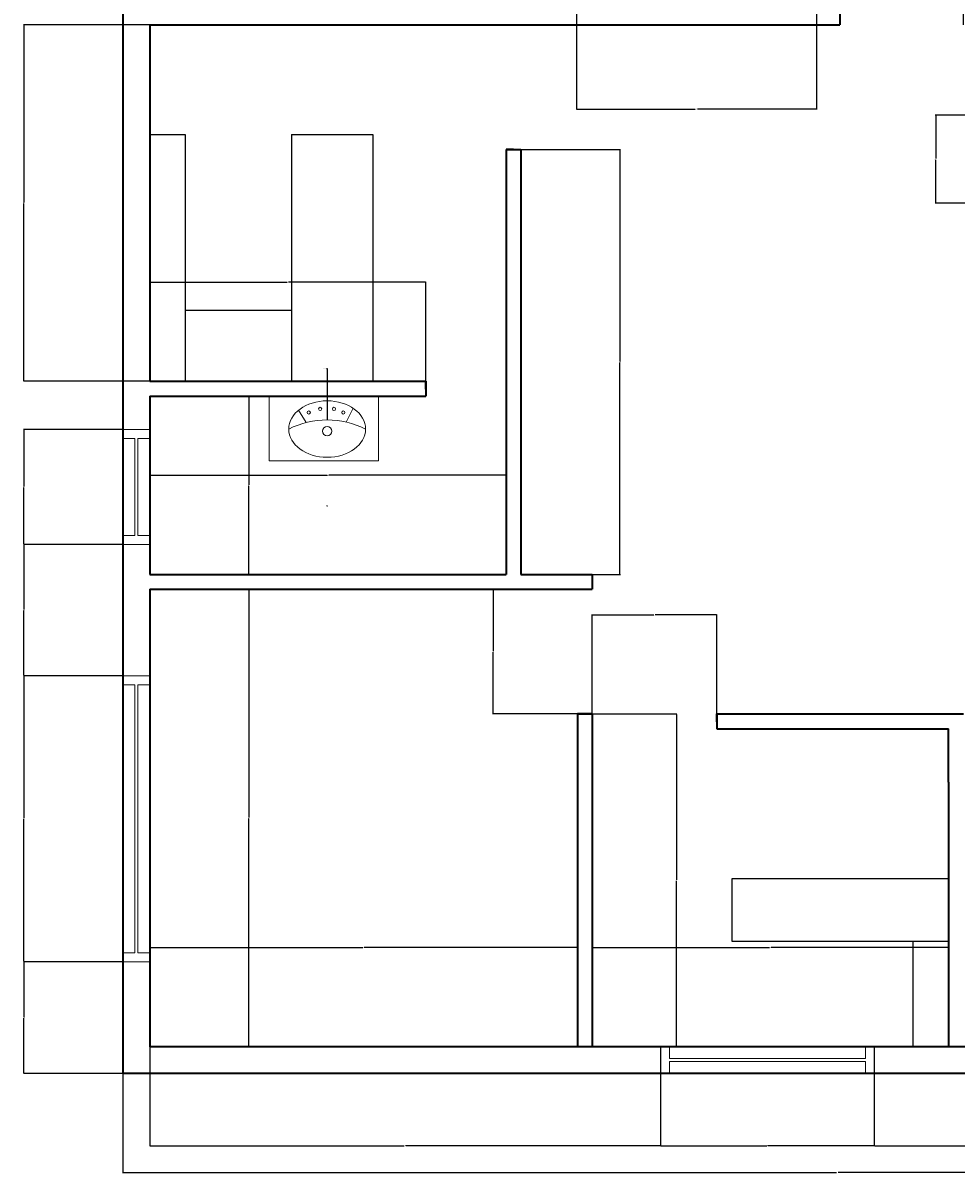
# Model space of a CAD drawing. Units: inches. Extents: x 1201 to 1750, y 1179 to 1858.
# Tile 1 of 3: x 1201 to 1515, y 1179 to 1566. Entities that reach past the tile are written whole.
import ezdxf

# ---------------------------------------------------------------- set-up
doc = ezdxf.new("R2010")
doc.units = ezdxf.units.IN
for name, color, linetype, lineweight in [('A-ANNO-DIMS', 2, 'Continuous', 18), ('A-FLOR-CASE', 9, 'Continuous', 25), ('A-FLOR-FIXT', 9, 'Continuous', 18), ('A-GLAZ', 4, 'Continuous', 18), ('A-WALL', 7, 'Continuous', 35)]:
    doc.layers.add(name, color=color, linetype=linetype, lineweight=lineweight)
doc.styles.get("Standard").update_dxf_attribs({"font": 'times.ttf'})
doc.dimstyles.get("Standard").update_dxf_attribs({"dimtxt": 0.18, "dimasz": 0.18, "dimexe": 0.18, "dimexo": 0.0625, "dimgap": 0.09, "dimtad": 0, "dimtih": 1, "dimtoh": 1, "dimdec": 4, "dimzin": 0, "dimdsep": 46, "dimtxsty": 'Standard', "dimcen": 0.09, "dimadec": 0, "dimazin": 0, "dimtfac": 1, "dimtdec": 4, "dimtofl": 0, "dimtmove": 0, "dimatfit": 3, "dimfxl": 1, "dimtolj": 1, "dimtzin": 0, "dimarcsym": 0})

# ---------------------------------------------------------------- blocks, each defined once
blk = doc.blocks.new('*D7')
at = {"layer": 'A-ANNO-DIMS', "color": 0, "lineweight": -2, "transparency": 16777216}
for p, q in [((1234.99, 1212.18), (1234.99, 1178.71)), ((1715.99, 1212.18), (1715.99, 1178.71)), ((1235.17, 1178.89), (1475.22, 1178.89)), ((1715.81, 1178.89), (1475.76, 1178.89))]:
    blk.add_line(p, q, dxfattribs=at)
at = {"layer": 'A-ANNO-DIMS', "color": 0, "transparency": 16777216}
for points in [[(1235.17, 1178.92), (1235.17, 1178.86), (1234.99, 1178.89)], [(1715.81, 1178.92), (1715.81, 1178.86), (1715.99, 1178.89)]]:
    blk.add_solid(points, dxfattribs=at)
at = {"layer": 'Defpoints', "color": 0, "transparency": 16777216}
for p in [(1234.99, 1212.24), (1715.99, 1212.24), (1234.99, 1178.89)]:
    blk.add_point(p, dxfattribs=at)
at = {"layer": 'A-ANNO-DIMS', "color": 0, "transparency": 16777216, "insert": (1475.49, 1178.89), "char_height": 0.18, "attachment_point": 5}
blk.add_mtext('\\A1;481', dxfattribs=at)
blk = doc.blocks.new('*D24')
at = {"layer": 'A-ANNO-DIMS', "color": 0, "lineweight": -2, "transparency": 16777216}
for p, q in [((1243.99, 1221.3), (1243.99, 1254.77)), ((1244.17, 1254.59), (1315.72, 1254.59)), ((1387.81, 1254.59), (1316.26, 1254.59)), ((1387.99, 1221.3), (1387.99, 1254.77))]:
    blk.add_line(p, q, dxfattribs=at)
at = {"layer": 'A-ANNO-DIMS', "color": 0, "transparency": 16777216}
for points in [[(1244.17, 1254.62), (1244.17, 1254.56), (1243.99, 1254.59)], [(1387.81, 1254.62), (1387.81, 1254.56), (1387.99, 1254.59)]]:
    blk.add_solid(points, dxfattribs=at)
at = {"layer": 'Defpoints', "color": 0, "transparency": 16777216}
for p in [(1387.99, 1254.59), (1243.99, 1221.24), (1387.99, 1221.24)]:
    blk.add_point(p, dxfattribs=at)
at = {"layer": 'A-ANNO-DIMS', "color": 0, "transparency": 16777216, "insert": (1315.99, 1254.59), "char_height": 0.18, "attachment_point": 5}
blk.add_mtext('\\A1;144', dxfattribs=at)
blk = doc.blocks.new('*D25')
at = {"layer": 'A-ANNO-DIMS', "color": 0, "lineweight": -2, "transparency": 16777216}
for p, q in [((1244.05, 1375.24), (1277.52, 1375.24)), ((1277.34, 1375.06), (1277.34, 1298.42)), ((1277.34, 1221.42), (1277.34, 1298.06)), ((1244.05, 1221.24), (1277.52, 1221.24))]:
    blk.add_line(p, q, dxfattribs=at)
at = {"layer": 'A-ANNO-DIMS', "color": 0, "transparency": 16777216}
for points in [[(1277.31, 1375.06), (1277.37, 1375.06), (1277.34, 1375.24)], [(1277.31, 1221.42), (1277.37, 1221.42), (1277.34, 1221.24)]]:
    blk.add_solid(points, dxfattribs=at)
at = {"layer": 'Defpoints', "color": 0, "transparency": 16777216}
for p in [(1243.99, 1375.24), (1243.99, 1221.24), (1277.34, 1221.24)]:
    blk.add_point(p, dxfattribs=at)
at = {"layer": 'A-ANNO-DIMS', "color": 0, "transparency": 16777216, "insert": (1277.34, 1298.24), "char_height": 0.18, "attachment_point": 5}
blk.add_mtext('\\A1;154', dxfattribs=at)
blk = doc.blocks.new('*D26')
at = {"layer": 'A-ANNO-DIMS', "color": 0, "lineweight": -2, "transparency": 16777216}
for p, q in [((1392.99, 1221.3), (1392.99, 1254.77)), ((1393.17, 1254.59), (1452.72, 1254.59)), ((1512.81, 1254.59), (1453.26, 1254.59)), ((1512.99, 1221.3), (1512.99, 1254.77))]:
    blk.add_line(p, q, dxfattribs=at)
at = {"layer": 'A-ANNO-DIMS', "color": 0, "transparency": 16777216}
for points in [[(1393.17, 1254.62), (1393.17, 1254.56), (1392.99, 1254.59)], [(1512.81, 1254.62), (1512.81, 1254.56), (1512.99, 1254.59)]]:
    blk.add_solid(points, dxfattribs=at)
at = {"layer": 'Defpoints', "color": 0, "transparency": 16777216}
for p in [(1512.99, 1254.59), (1392.99, 1221.24), (1512.99, 1221.24)]:
    blk.add_point(p, dxfattribs=at)
at = {"layer": 'A-ANNO-DIMS', "color": 0, "transparency": 16777216, "insert": (1452.99, 1254.59), "char_height": 0.18, "attachment_point": 5}
blk.add_mtext('\\A1;120', dxfattribs=at)
blk = doc.blocks.new('*D27')
at = {"layer": 'A-ANNO-DIMS', "color": 0, "lineweight": -2, "transparency": 16777216}
for p, q in [((1388.049469, 1333.241877), (1421.516969, 1333.241877)), ((1421.336969, 1333.061877), (1421.336969, 1277.421877)), ((1421.336969, 1221.421877), (1421.336969, 1277.061877)), ((1388.049469, 1221.241877), (1421.516969, 1221.241877))]:
    blk.add_line(p, q, dxfattribs=at)
at = {"layer": 'A-ANNO-DIMS', "color": 0, "transparency": 16777216}
for points in [[(1421.306969, 1333.061877), (1421.366969, 1333.061877), (1421.336969, 1333.241877)], [(1421.306969, 1221.421877), (1421.366969, 1221.421877), (1421.336969, 1221.241877)]]:
    blk.add_solid(points, dxfattribs=at)
at = {"layer": 'Defpoints', "color": 0, "transparency": 16777216}
for p in [(1387.986969, 1333.241877), (1387.986969, 1221.241877), (1421.336969, 1221.241877)]:
    blk.add_point(p, dxfattribs=at)
at = {"layer": 'A-ANNO-DIMS', "color": 0, "transparency": 16777216, "insert": (1421.336969, 1277.241877), "char_height": 0.18, "attachment_point": 5}
blk.add_mtext('\\A1;112', dxfattribs=at)
blk = doc.blocks.new('*D28')
at = {"layer": 'A-ANNO-DIMS', "color": 0, "lineweight": -2, "transparency": 16777216}
for p, q in [((1243.99, 1380.3), (1243.99, 1413.77)), ((1244.17, 1413.59), (1303.72, 1413.59)), ((1363.81, 1413.59), (1304.26, 1413.59)), ((1363.99, 1380.3), (1363.99, 1413.77))]:
    blk.add_line(p, q, dxfattribs=at)
at = {"layer": 'A-ANNO-DIMS', "color": 0, "transparency": 16777216}
for points in [[(1244.17, 1413.62), (1244.17, 1413.56), (1243.99, 1413.59)], [(1363.81, 1413.62), (1363.81, 1413.56), (1363.99, 1413.59)]]:
    blk.add_solid(points, dxfattribs=at)
at = {"layer": 'Defpoints', "color": 0, "transparency": 16777216}
for p in [(1363.99, 1413.59), (1243.99, 1380.24), (1363.99, 1380.24)]:
    blk.add_point(p, dxfattribs=at)
at = {"layer": 'A-ANNO-DIMS', "color": 0, "transparency": 16777216, "insert": (1303.99, 1413.59), "char_height": 0.18, "attachment_point": 5}
blk.add_mtext('\\A1;120', dxfattribs=at)
blk = doc.blocks.new('*D29')
at = {"layer": 'A-ANNO-DIMS', "color": 0, "lineweight": -2, "transparency": 16777216}
for p, q in [((1244.05, 1440.24), (1277.52, 1440.24)), ((1277.34, 1440.06), (1277.34, 1410.42)), ((1277.34, 1380.42), (1277.34, 1410.06)), ((1244.05, 1380.24), (1277.52, 1380.24))]:
    blk.add_line(p, q, dxfattribs=at)
at = {"layer": 'A-ANNO-DIMS', "color": 0, "transparency": 16777216}
for points in [[(1277.31, 1440.06), (1277.37, 1440.06), (1277.34, 1440.24)], [(1277.31, 1380.42), (1277.37, 1380.42), (1277.34, 1380.24)]]:
    blk.add_solid(points, dxfattribs=at)
at = {"layer": 'Defpoints', "color": 0, "transparency": 16777216}
for p in [(1243.99, 1440.24), (1243.99, 1380.24), (1277.34, 1380.24)]:
    blk.add_point(p, dxfattribs=at)
at = {"layer": 'A-ANNO-DIMS', "color": 0, "transparency": 16777216, "insert": (1277.34, 1410.24), "char_height": 0.18, "attachment_point": 5}
blk.add_mtext('\\A1;60', dxfattribs=at)
blk = doc.blocks.new('*D30')
at = {"layer": 'A-ANNO-DIMS', "color": 0, "lineweight": -2, "transparency": 16777216}
for p, q in [((1243.92, 1565.24), (1201.46, 1565.24)), ((1201.64, 1565.06), (1201.64, 1505.42)), ((1201.64, 1445.42), (1201.64, 1505.06)), ((1243.92, 1445.24), (1201.46, 1445.24))]:
    blk.add_line(p, q, dxfattribs=at)
at = {"layer": 'A-ANNO-DIMS', "color": 0, "transparency": 16777216}
for points in [[(1201.61, 1565.06), (1201.67, 1565.06), (1201.64, 1565.24)], [(1201.61, 1445.42), (1201.67, 1445.42), (1201.64, 1445.24)]]:
    blk.add_solid(points, dxfattribs=at)
at = {"layer": 'Defpoints', "color": 0, "transparency": 16777216}
for p in [(1201.64, 1565.24), (1243.99, 1565.24), (1243.99, 1445.24)]:
    blk.add_point(p, dxfattribs=at)
at = {"layer": 'A-ANNO-DIMS', "color": 0, "transparency": 16777216, "insert": (1201.64, 1505.24), "char_height": 0.18, "attachment_point": 5}
blk.add_mtext('\\A1;120', dxfattribs=at)
blk = doc.blocks.new('*D33')
at = {"layer": 'A-ANNO-DIMS', "color": 0, "lineweight": -2, "transparency": 16777216}
for p, q in [((1476.42, 1565.3), (1476.42, 1598.77)), ((1476.6, 1598.59), (1496.82, 1598.59)), ((1517.81, 1598.59), (1497.58, 1598.59)), ((1517.99, 1565.3), (1517.99, 1598.77))]:
    blk.add_line(p, q, dxfattribs=at)
at = {"layer": 'A-ANNO-DIMS', "color": 0, "transparency": 16777216}
for points in [[(1476.6, 1598.62), (1476.6, 1598.56), (1476.42, 1598.59)], [(1517.81, 1598.62), (1517.81, 1598.56), (1517.99, 1598.59)]]:
    blk.add_solid(points, dxfattribs=at)
at = {"layer": 'Defpoints', "color": 0, "transparency": 16777216}
for p in [(1517.99, 1598.59), (1476.42, 1565.24), (1517.99, 1565.24)]:
    blk.add_point(p, dxfattribs=at)
at = {"layer": 'A-ANNO-DIMS', "color": 0, "transparency": 16777216, "insert": (1497.2, 1598.59), "char_height": 0.18, "attachment_point": 5}
blk.add_mtext('\\A1;41.57', dxfattribs=at)
blk = doc.blocks.new('*D36')
at = {"layer": 'A-ANNO-DIMS', "color": 0, "lineweight": -2, "transparency": 16777216}
for p, q in [((1234.92, 1249.83), (1201.46, 1249.83)), ((1201.64, 1249.65), (1201.64, 1231.22)), ((1201.64, 1212.42), (1201.64, 1230.86)), ((1234.92, 1212.24), (1201.46, 1212.24))]:
    blk.add_line(p, q, dxfattribs=at)
at = {"layer": 'A-ANNO-DIMS', "color": 0, "transparency": 16777216}
for points in [[(1201.61, 1249.65), (1201.67, 1249.65), (1201.64, 1249.83)], [(1201.61, 1212.42), (1201.67, 1212.42), (1201.64, 1212.24)]]:
    blk.add_solid(points, dxfattribs=at)
at = {"layer": 'Defpoints', "color": 0, "transparency": 16777216}
for p in [(1201.64, 1249.83), (1234.99, 1249.83), (1234.99, 1212.24)]:
    blk.add_point(p, dxfattribs=at)
at = {"layer": 'A-ANNO-DIMS', "color": 0, "transparency": 16777216, "insert": (1201.64, 1231.04), "char_height": 0.18, "attachment_point": 5}
blk.add_mtext('\\A1;37.59', dxfattribs=at)
blk = doc.blocks.new('*D37')
at = {"layer": 'A-ANNO-DIMS', "color": 0, "lineweight": -2, "transparency": 16777216}
for p, q in [((1234.92, 1346.08), (1201.46, 1346.08)), ((1201.64, 1345.9), (1201.64, 1298.14)), ((1201.64, 1250.01), (1201.64, 1297.78)), ((1234.92, 1249.83), (1201.46, 1249.83))]:
    blk.add_line(p, q, dxfattribs=at)
at = {"layer": 'A-ANNO-DIMS', "color": 0, "transparency": 16777216}
for points in [[(1201.61, 1345.9), (1201.67, 1345.9), (1201.64, 1346.08)], [(1201.61, 1250.01), (1201.67, 1250.01), (1201.64, 1249.83)]]:
    blk.add_solid(points, dxfattribs=at)
at = {"layer": 'Defpoints', "color": 0, "transparency": 16777216}
for p in [(1201.64, 1346.08), (1234.99, 1346.08), (1234.99, 1249.83)]:
    blk.add_point(p, dxfattribs=at)
at = {"layer": 'A-ANNO-DIMS', "color": 0, "transparency": 16777216, "insert": (1201.64, 1297.96), "char_height": 0.18, "attachment_point": 5}
blk.add_mtext('\\A1;96.25', dxfattribs=at)
blk = doc.blocks.new('*D38')
at = {"layer": 'A-ANNO-DIMS', "color": 0, "lineweight": -2, "transparency": 16777216}
for p, q in [((1234.92, 1390.34), (1201.46, 1390.34)), ((1201.64, 1390.16), (1201.64, 1368.39)), ((1201.64, 1346.26), (1201.64, 1368.03)), ((1234.92, 1346.08), (1201.46, 1346.08))]:
    blk.add_line(p, q, dxfattribs=at)
at = {"layer": 'A-ANNO-DIMS', "color": 0, "transparency": 16777216}
for points in [[(1201.61, 1390.16), (1201.67, 1390.16), (1201.64, 1390.34)], [(1201.61, 1346.26), (1201.67, 1346.26), (1201.64, 1346.08)]]:
    blk.add_solid(points, dxfattribs=at)
at = {"layer": 'Defpoints', "color": 0, "transparency": 16777216}
for p in [(1201.64, 1390.34), (1234.99, 1390.34), (1234.99, 1346.08)]:
    blk.add_point(p, dxfattribs=at)
at = {"layer": 'A-ANNO-DIMS', "color": 0, "transparency": 16777216, "insert": (1201.64, 1368.21), "char_height": 0.18, "attachment_point": 5}
blk.add_mtext('\\A1;44.26', dxfattribs=at)
blk = doc.blocks.new('*D39')
at = {"layer": 'A-ANNO-DIMS', "color": 0, "lineweight": -2, "transparency": 16777216}
for p, q in [((1234.92, 1428.98), (1201.46, 1428.98)), ((1201.64, 1428.8), (1201.64, 1409.84)), ((1201.64, 1390.52), (1201.64, 1409.48)), ((1234.92, 1390.34), (1201.46, 1390.34))]:
    blk.add_line(p, q, dxfattribs=at)
at = {"layer": 'A-ANNO-DIMS', "color": 0, "transparency": 16777216}
for points in [[(1201.61, 1428.8), (1201.67, 1428.8), (1201.64, 1428.98)], [(1201.61, 1390.52), (1201.67, 1390.52), (1201.64, 1390.34)]]:
    blk.add_solid(points, dxfattribs=at)
at = {"layer": 'Defpoints', "color": 0, "transparency": 16777216}
for p in [(1201.64, 1428.98), (1234.99, 1428.98), (1234.99, 1390.34)]:
    blk.add_point(p, dxfattribs=at)
at = {"layer": 'A-ANNO-DIMS', "color": 0, "transparency": 16777216, "insert": (1201.64, 1409.66), "char_height": 0.18, "attachment_point": 5}
blk.add_mtext('\\A1;38.64', dxfattribs=at)
blk = doc.blocks.new('*D40')
at = {"layer": 'A-ANNO-DIMS', "color": 0, "lineweight": -2, "transparency": 16777216}
for p, q in [((1243.99, 1221.18), (1243.99, 1187.71)), ((1415.97, 1221.18), (1415.97, 1187.71)), ((1244.17, 1187.89), (1329.71, 1187.89)), ((1415.79, 1187.89), (1330.25, 1187.89))]:
    blk.add_line(p, q, dxfattribs=at)
at = {"layer": 'A-ANNO-DIMS', "color": 0, "transparency": 16777216}
for points in [[(1244.17, 1187.92), (1244.17, 1187.86), (1243.99, 1187.89)], [(1415.79, 1187.92), (1415.79, 1187.86), (1415.97, 1187.89)]]:
    blk.add_solid(points, dxfattribs=at)
at = {"layer": 'Defpoints', "color": 0, "transparency": 16777216}
for p in [(1243.99, 1221.24), (1415.97, 1221.24), (1243.99, 1187.89)]:
    blk.add_point(p, dxfattribs=at)
at = {"layer": 'A-ANNO-DIMS', "color": 0, "transparency": 16777216, "insert": (1329.98, 1187.89), "char_height": 0.18, "attachment_point": 5}
blk.add_mtext('\\A1;172', dxfattribs=at)
blk = doc.blocks.new('*D41')
at = {"layer": 'A-ANNO-DIMS', "color": 0, "lineweight": -2, "transparency": 16777216}
for p, q in [((1415.97, 1221.18), (1415.97, 1187.71)), ((1487.97, 1221.18), (1487.97, 1187.71)), ((1416.15, 1187.89), (1451.76, 1187.89)), ((1487.79, 1187.89), (1452.18, 1187.89))]:
    blk.add_line(p, q, dxfattribs=at)
at = {"layer": 'A-ANNO-DIMS', "color": 0, "transparency": 16777216}
for points in [[(1416.15, 1187.92), (1416.15, 1187.86), (1415.97, 1187.89)], [(1487.79, 1187.92), (1487.79, 1187.86), (1487.97, 1187.89)]]:
    blk.add_solid(points, dxfattribs=at)
at = {"layer": 'Defpoints', "color": 0, "transparency": 16777216}
for p in [(1415.97, 1221.24), (1487.97, 1221.24), (1415.97, 1187.89)]:
    blk.add_point(p, dxfattribs=at)
at = {"layer": 'A-ANNO-DIMS', "color": 0, "transparency": 16777216, "insert": (1451.97, 1187.89), "char_height": 0.18, "attachment_point": 5}
blk.add_mtext('\\A1;72', dxfattribs=at)
blk = doc.blocks.new('*D42')
at = {"layer": 'A-ANNO-DIMS', "color": 0, "lineweight": -2, "transparency": 16777216}
for p, q in [((1487.97, 1221.18), (1487.97, 1187.71)), ((1551.45, 1221.18), (1551.45, 1187.71)), ((1488.15, 1187.89), (1519.33, 1187.89)), ((1551.27, 1187.89), (1520.09, 1187.89))]:
    blk.add_line(p, q, dxfattribs=at)
at = {"layer": 'A-ANNO-DIMS', "color": 0, "transparency": 16777216}
for points in [[(1488.15, 1187.92), (1488.15, 1187.86), (1487.97, 1187.89)], [(1551.27, 1187.92), (1551.27, 1187.86), (1551.45, 1187.89)]]:
    blk.add_solid(points, dxfattribs=at)
at = {"layer": 'Defpoints', "color": 0, "transparency": 16777216}
for p in [(1487.97, 1221.24), (1551.45, 1221.24), (1487.97, 1187.89)]:
    blk.add_point(p, dxfattribs=at)
at = {"layer": 'A-ANNO-DIMS', "color": 0, "transparency": 16777216, "insert": (1519.71, 1187.89), "char_height": 0.18, "attachment_point": 5}
blk.add_mtext('\\A1;63.48', dxfattribs=at)
blk = doc.blocks.new('*D45')
at = {"layer": 'A-ANNO-DIMS', "color": 0, "lineweight": -2, "transparency": 16777216}
for p, q in [((1369.05, 1523.24), (1402.52, 1523.24)), ((1402.34, 1523.06), (1402.34, 1451.92)), ((1402.34, 1380.42), (1402.34, 1451.56)), ((1369.05, 1380.24), (1402.52, 1380.24))]:
    blk.add_line(p, q, dxfattribs=at)
at = {"layer": 'A-ANNO-DIMS', "color": 0, "transparency": 16777216}
for points in [[(1402.31, 1523.06), (1402.37, 1523.06), (1402.34, 1523.24)], [(1402.31, 1380.42), (1402.37, 1380.42), (1402.34, 1380.24)]]:
    blk.add_solid(points, dxfattribs=at)
at = {"layer": 'Defpoints', "color": 0, "transparency": 16777216}
for p in [(1368.99, 1523.24), (1368.99, 1380.24), (1402.34, 1380.24)]:
    blk.add_point(p, dxfattribs=at)
at = {"layer": 'A-ANNO-DIMS', "color": 0, "transparency": 16777216, "insert": (1402.34, 1451.74), "char_height": 0.18, "attachment_point": 5}
blk.add_mtext('\\A1;143', dxfattribs=at)
blk = doc.blocks.new('*D46')
at = {"layer": 'A-ANNO-DIMS', "color": 0, "lineweight": -2, "transparency": 16777216}
for p, q in [((1392.99, 1333.3), (1392.99, 1366.77)), ((1434.99, 1333.3), (1434.99, 1366.77)), ((1393.17, 1366.59), (1413.77, 1366.59)), ((1434.81, 1366.59), (1414.2, 1366.59))]:
    blk.add_line(p, q, dxfattribs=at)
at = {"layer": 'A-ANNO-DIMS', "color": 0, "transparency": 16777216}
for points in [[(1393.17, 1366.62), (1393.17, 1366.56), (1392.99, 1366.59)], [(1434.81, 1366.62), (1434.81, 1366.56), (1434.99, 1366.59)]]:
    blk.add_solid(points, dxfattribs=at)
at = {"layer": 'Defpoints', "color": 0, "transparency": 16777216}
for p in [(1434.99, 1366.59), (1392.99, 1333.24), (1434.99, 1333.24)]:
    blk.add_point(p, dxfattribs=at)
at = {"layer": 'A-ANNO-DIMS', "color": 0, "transparency": 16777216, "insert": (1413.99, 1366.59), "char_height": 0.18, "attachment_point": 5}
blk.add_mtext('\\A1;42', dxfattribs=at)
blk = doc.blocks.new('*D47')
at = {"layer": 'A-ANNO-DIMS', "color": 0, "lineweight": -2, "transparency": 16777216}
for p, q in [((1392.924469, 1375.241877), (1359.456969, 1375.241877)), ((1359.636969, 1375.061877), (1359.636969, 1354.421877)), ((1359.636969, 1333.421877), (1359.636969, 1354.061877)), ((1392.924469, 1333.241877), (1359.456969, 1333.241877))]:
    blk.add_line(p, q, dxfattribs=at)
at = {"layer": 'A-ANNO-DIMS', "color": 0, "transparency": 16777216}
for points in [[(1359.606969, 1375.061877), (1359.666969, 1375.061877), (1359.636969, 1375.241877)], [(1359.606969, 1333.421877), (1359.666969, 1333.421877), (1359.636969, 1333.241877)]]:
    blk.add_solid(points, dxfattribs=at)
at = {"layer": 'Defpoints', "color": 0, "transparency": 16777216}
for p in [(1359.636969, 1375.241877), (1392.986969, 1375.241877), (1392.986969, 1333.241877)]:
    blk.add_point(p, dxfattribs=at)
at = {"layer": 'A-ANNO-DIMS', "color": 0, "transparency": 16777216, "insert": (1359.636969, 1354.241877), "char_height": 0.18, "attachment_point": 5}
blk.add_mtext('\\A1;42', dxfattribs=at)
blk = doc.blocks.new('*D50')
at = {"layer": 'A-ANNO-DIMS', "color": 0, "lineweight": -2, "transparency": 16777216}
for p, q in [((1541.92, 1534.83), (1508.46, 1534.83)), ((1508.64, 1534.65), (1508.64, 1520.22)), ((1508.64, 1505.42), (1508.64, 1519.85)), ((1541.92, 1505.24), (1508.46, 1505.24))]:
    blk.add_line(p, q, dxfattribs=at)
at = {"layer": 'A-ANNO-DIMS', "color": 0, "transparency": 16777216}
for points in [[(1508.61, 1534.65), (1508.67, 1534.65), (1508.64, 1534.83)], [(1508.61, 1505.42), (1508.67, 1505.42), (1508.64, 1505.24)]]:
    blk.add_solid(points, dxfattribs=at)
at = {"layer": 'Defpoints', "color": 0, "transparency": 16777216}
for p in [(1508.64, 1534.83), (1541.99, 1534.83), (1541.99, 1505.24)]:
    blk.add_point(p, dxfattribs=at)
at = {"layer": 'A-ANNO-DIMS', "color": 0, "transparency": 16777216, "insert": (1508.64, 1520.03), "char_height": 0.18, "attachment_point": 5}
blk.add_mtext('\\A1;29.585', dxfattribs=at)
blk = doc.blocks.new('*D59')
at = {"layer": 'A-ANNO-DIMS', "color": 0, "lineweight": -2, "transparency": 16777216}
for p, q in [((1243.99, 1445.3), (1243.99, 1478.77)), ((1244.17, 1478.59), (1290.28, 1478.59)), ((1336.81, 1478.59), (1290.69, 1478.59)), ((1336.99, 1445.3), (1336.99, 1478.77))]:
    blk.add_line(p, q, dxfattribs=at)
at = {"layer": 'A-ANNO-DIMS', "color": 0, "transparency": 16777216}
for points in [[(1244.17, 1478.62), (1244.17, 1478.56), (1243.99, 1478.59)], [(1336.81, 1478.62), (1336.81, 1478.56), (1336.99, 1478.59)]]:
    blk.add_solid(points, dxfattribs=at)
at = {"layer": 'Defpoints', "color": 0, "transparency": 16777216}
for p in [(1336.99, 1478.59), (1243.99, 1445.24), (1336.99, 1445.24)]:
    blk.add_point(p, dxfattribs=at)
at = {"layer": 'A-ANNO-DIMS', "color": 0, "transparency": 16777216, "insert": (1290.49, 1478.59), "char_height": 0.18, "attachment_point": 5}
blk.add_mtext('\\A1;93', dxfattribs=at)
blk = doc.blocks.new('*D62')
at = {"layer": 'A-ANNO-DIMS', "color": 0, "lineweight": -2, "transparency": 16777216}
for p, q in [((1387.67, 1570.18), (1387.67, 1536.71)), ((1468.48, 1570.18), (1468.48, 1536.71)), ((1387.85, 1536.89), (1427.71, 1536.89)), ((1468.3, 1536.89), (1428.44, 1536.89))]:
    blk.add_line(p, q, dxfattribs=at)
at = {"layer": 'A-ANNO-DIMS', "color": 0, "transparency": 16777216}
for points in [[(1387.85, 1536.92), (1387.85, 1536.86), (1387.67, 1536.89)], [(1468.3, 1536.92), (1468.3, 1536.86), (1468.48, 1536.89)]]:
    blk.add_solid(points, dxfattribs=at)
at = {"layer": 'Defpoints', "color": 0, "transparency": 16777216}
for p in [(1387.67, 1570.24), (1468.48, 1570.24), (1387.67, 1536.89)]:
    blk.add_point(p, dxfattribs=at)
at = {"layer": 'A-ANNO-DIMS', "color": 0, "transparency": 16777216, "insert": (1428.07, 1536.89), "char_height": 0.18, "attachment_point": 5}
blk.add_mtext('\\A1;80.81', dxfattribs=at)
blk = doc.blocks.new('*D63')
at = {"layer": 'A-ANNO-DIMS', "color": 0, "lineweight": -2, "transparency": 16777216}
for p, q in [((1303.57, 1449.56), (1303.75, 1449.56)), ((1303.75, 1449.56), (1303.75, 1432.41)), ((1303.66, 1403.35), (1303.84, 1403.35)), ((1303.75, 1403.26), (1303.75, 1403.44))]:
    blk.add_line(p, q, dxfattribs=at)
at = {"layer": 'A-ANNO-DIMS', "color": 0, "transparency": 16777216}
blk.add_solid([(1303.78, 1432.41), (1303.72, 1432.41), (1303.75, 1432.23)], dxfattribs=at)
at = {"layer": 'Defpoints', "color": 0, "transparency": 16777216}
for p in [(1303.75, 1432.23), (1303.75, 1403.35)]:
    blk.add_point(p, dxfattribs=at)
at = {"layer": 'A-ANNO-DIMS', "color": 0, "transparency": 16777216, "insert": (1303.03, 1449.56), "char_height": 0.18, "attachment_point": 5}
blk.add_mtext('\\A1;R28.884', dxfattribs=at)

msp = doc.modelspace()

# ---------------------------------------------------------------- linework, layer by layer
at = {"layer": 'A-FLOR-CASE'}
for p, q in [((1243.987, 1528.3245), (1255.987, 1528.3245)), ((1255.987, 1528.3245), (1255.987, 1445.2419)), ((1291.795, 1528.3245), (1291.795, 1445.2419)), ((1291.795, 1528.3245), (1319.1055, 1528.3245)), ((1319.1055, 1528.3245), (1319.1055, 1445.2419)), ((1255.987, 1469.2419), (1291.795, 1469.2419)), ((1440.0853, 1256.6537), (1440.0853, 1277.8567)), ((1440.0853, 1277.8567), (1512.987, 1277.8567)), ((1512.987, 1256.6537), (1440.0853, 1256.6537)), ((1500.987, 1256.6537), (1500.987, 1221.2419))]:
    msp.add_line(p, q, dxfattribs=at)
at = {"layer": 'A-FLOR-FIXT'}
for p, q in [((1284.2092, 1440.2419), (1284.2092, 1418.4305)), ((1321.0174, 1418.4305), (1321.0174, 1440.2419)), ((1294.0555, 1435.4667), (1296.6227, 1431.3364)), ((1312.538, 1436.1462), (1310.1246, 1431.5165)), ((1310.1246, 1431.5165), (1310.1246, 1431.5165)), ((1284.2092, 1418.4305), (1321.0174, 1418.4305))]:
    msp.add_line(p, q, dxfattribs=at)
for centre, radius in [((1301.3932, 1435.934), 0.5463), ((1306.0404, 1435.9602), 0.5463), ((1297.5571, 1434.7303), 0.5463), ((1309.1801, 1434.7303), 0.5463), ((1303.7483, 1428.4525), 1.5789)]:
    msp.add_circle(centre, radius, dxfattribs=at)
msp.add_arc((1303.7483, 1403.3453), 28.8837, 63.395862, 116.604138, dxfattribs=at)
msp.add_ellipse((1303.7483, 1429.1709), major_axis=(-12.9348, 0), ratio=0.73505504, dxfattribs=at)
at = {"layer": 'A-GLAZ'}
for p, q in [((1234.987, 1428.9844), (1243.987, 1428.9844)), ((1234.987, 1425.9844), (1238.987, 1425.9844)), ((1238.987, 1425.9844), (1238.987, 1393.3406)), ((1239.987, 1425.9844), (1239.987, 1393.3406)), ((1239.987, 1425.9844), (1243.987, 1425.9844)), ((1234.987, 1393.3406), (1238.987, 1393.3406)), ((1239.487, 1390.3406), (1234.987, 1390.3406)), ((1234.987, 1390.3406), (1243.987, 1390.3406)), ((1239.987, 1393.3406), (1243.987, 1393.3406)), ((1234.987, 1346.0807), (1243.987, 1346.0807)), ((1234.987, 1343.0807), (1238.987, 1343.0807)), ((1238.987, 1343.0807), (1238.987, 1252.8345)), ((1239.987, 1343.0807), (1239.987, 1252.8345)), ((1239.987, 1343.0807), (1243.987, 1343.0807)), ((1234.987, 1252.8345), (1238.987, 1252.8345)), ((1239.987, 1252.8345), (1243.987, 1252.8345)), ((1234.987, 1249.8345), (1243.987, 1249.8345)), ((1415.9712, 1221.2419), (1415.9712, 1212.2419)), ((1418.9712, 1221.2419), (1418.9712, 1217.2419)), ((1484.9712, 1221.2419), (1484.9712, 1217.2419)), ((1487.9712, 1216.7419), (1487.9712, 1221.2419)), ((1487.9712, 1221.2419), (1487.9712, 1212.2419)), ((1418.9712, 1217.2419), (1484.9712, 1217.2419)), ((1418.9712, 1216.2419), (1484.9712, 1216.2419)), ((1418.9712, 1216.2419), (1418.9712, 1212.2419)), ((1484.9712, 1216.2419), (1484.9712, 1212.2419))]:
    msp.add_line(p, q, dxfattribs=at)
at = {"layer": 'A-WALL'}
for p, q in [((1234.987, 1711.2419), (1234.987, 1222.2419)), ((1476.4162, 1570.2419), (1476.4162, 1565.2419)), ((1243.987, 1565.2419), (1476.4162, 1565.2419)), ((1243.987, 1565.2419), (1243.987, 1445.2419)), ((1363.987, 1523.2419), (1363.987, 1380.2419)), ((1363.987, 1523.2419), (1363.987, 1380.2419)), ((1366.4338, 1523.2419), (1363.987, 1523.2419)), ((1363.987, 1523.2419), (1368.987, 1523.2419)), ((1368.987, 1523.2419), (1368.987, 1380.2419)), ((1368.987, 1523.2419), (1368.987, 1380.2419)), ((1243.987, 1445.2419), (1336.987, 1445.2419)), ((1336.987, 1442.5492), (1336.987, 1445.2419)), ((1336.987, 1445.2419), (1336.987, 1440.2419)), ((1243.987, 1440.2419), (1336.987, 1440.2419)), ((1243.987, 1440.2419), (1243.987, 1380.2419)), ((1243.987, 1380.2419), (1363.987, 1380.2419)), ((1368.987, 1380.2419), (1392.987, 1380.2419)), ((1392.987, 1380.2419), (1392.987, 1375.2419)), ((1243.987, 1375.2419), (1392.987, 1375.2419)), ((1243.987, 1375.2419), (1243.987, 1231.2419)), ((1392.987, 1333.2419), (1387.987, 1333.2419)), ((1387.987, 1333.2419), (1392.987, 1333.2419)), ((1387.987, 1333.2419), (1387.987, 1221.2419)), ((1392.987, 1333.2419), (1392.987, 1221.2419)), ((1434.987, 1330.5878), (1434.987, 1333.2419)), ((1434.987, 1333.2419), (1434.987, 1328.2419)), ((1434.987, 1333.2419), (1517.987, 1333.2419)), ((1434.987, 1328.2419), (1512.987, 1328.2419)), ((1512.987, 1310.2419), (1512.987, 1328.2419)), ((1512.987, 1310.2419), (1512.987, 1221.2419)), ((1243.987, 1231.2419), (1243.987, 1221.2419)), ((1234.987, 1222.2419), (1234.987, 1212.2419)), ((1706.987, 1221.2419), (1243.987, 1221.2419)), ((1715.987, 1212.2419), (1234.987, 1212.2419))]:
    msp.add_line(p, q, dxfattribs=at)

# ---------------------------------------------------------------- dimensions: what is measured, and where the dimension line sits
at = {"layer": 'A-ANNO-DIMS'}
for base, p1, p2, override, picture, middle in [((1517.987, 1598.5919), (1476.4162, 1565.2419), (1517.987, 1565.2419), {"dimdec": 2, "dimlfac": 1, "dimrnd": 0, "dimzin": 0, "dimdsep": 46, "dimlunit": 2}, '*D33', (1497.2016, 1598.5919)), ((1336.987, 1478.5919), (1243.987, 1445.2419), (1336.987, 1445.2419), {"dimdec": 0, "dimlfac": 1, "dimrnd": 0, "dimzin": 0, "dimdsep": 46, "dimlunit": 2}, '*D59', (1290.487, 1478.5919)), ((1363.987, 1413.5919), (1243.987, 1380.2419), (1363.987, 1380.2419), {"dimdec": 0, "dimlfac": 1, "dimrnd": 0, "dimzin": 0, "dimdsep": 46, "dimlunit": 2}, '*D28', (1303.987, 1413.5919)), ((1434.987, 1366.5919), (1392.987, 1333.2419), (1434.987, 1333.2419), {"dimdec": 0, "dimlfac": 1, "dimrnd": 0, "dimzin": 0, "dimdsep": 46, "dimlunit": 2}, '*D46', (1413.987, 1366.5919)), ((1512.987, 1254.5919), (1392.987, 1221.2419), (1512.987, 1221.2419), {"dimdec": 0, "dimlfac": 1, "dimrnd": 0, "dimzin": 0, "dimdsep": 46, "dimlunit": 2}, '*D26', (1452.987, 1254.5919))]:
    dim = msp.add_linear_dim(base=base, p1=p1, p2=p2, dimstyle='Standard', override=override, dxfattribs=at)
    dim.commit()
    dim.dimension.update_dxf_attribs({"geometry": picture, "text_midpoint": middle})
for base, p1, p2, angle, override, picture, middle in [((1387.6681, 1536.8919), (1468.4762, 1570.2419), (1387.6681, 1570.2419), 180, {"dimdec": 2, "dimlfac": 1, "dimrnd": 0, "dimzin": 0, "dimdsep": 46, "dimlunit": 2}, '*D62', (1428.0721, 1536.8919)), ((1201.637, 1565.2419), (1243.987, 1445.2419), (1243.987, 1565.2419), 90, {"dimdec": 0, "dimlfac": 1, "dimrnd": 0, "dimzin": 0, "dimdsep": 46, "dimlunit": 2}, '*D30', (1201.637, 1505.2419)), ((1508.637, 1534.8271), (1541.987, 1505.2419), (1541.987, 1534.8271), 90, {"dimdec": 3, "dimlfac": 1, "dimrnd": 0, "dimzin": 0, "dimdsep": 46, "dimlunit": 2}, '*D50', (1508.637, 1520.0345)), ((1402.337, 1380.2419), (1368.987, 1523.2419), (1368.987, 1380.2419), 270, {"dimdec": 0, "dimlfac": 1, "dimrnd": 0, "dimzin": 0, "dimdsep": 46, "dimlunit": 2}, '*D45', (1402.337, 1451.7419)), ((1277.337, 1380.2419), (1243.987, 1440.2419), (1243.987, 1380.2419), 270, {"dimdec": 0, "dimlfac": 1, "dimrnd": 0, "dimzin": 0, "dimdsep": 46, "dimlunit": 2}, '*D29', (1277.337, 1410.2419)), ((1201.637, 1428.9844), (1234.987, 1390.3406), (1234.987, 1428.9844), 90, {"dimdec": 2, "dimlfac": 1, "dimrnd": 0, "dimzin": 0, "dimdsep": 46, "dimlunit": 2}, '*D39', (1201.637, 1409.6625)), ((1201.637, 1390.3406), (1234.987, 1346.0807), (1234.987, 1390.3406), 90, {"dimdec": 2, "dimlfac": 1, "dimrnd": 0, "dimzin": 0, "dimdsep": 46, "dimlunit": 2}, '*D38', (1201.637, 1368.2107)), ((1277.337, 1221.2419), (1243.987, 1375.2419), (1243.987, 1221.2419), 270, {"dimdec": 0, "dimlfac": 1, "dimrnd": 0, "dimzin": 0, "dimdsep": 46, "dimlunit": 2}, '*D25', (1277.337, 1298.2419)), ((1359.637, 1375.2419), (1392.987, 1333.2419), (1392.987, 1375.2419), 90, {"dimdec": 0, "dimlfac": 1, "dimrnd": 0, "dimzin": 0, "dimdsep": 46, "dimlunit": 2}, '*D47', (1359.637, 1354.2419)), ((1201.637, 1346.0807), (1234.987, 1249.8345), (1234.987, 1346.0807), 90, {"dimdec": 2, "dimlfac": 1, "dimrnd": 0, "dimzin": 0, "dimdsep": 46, "dimlunit": 2}, '*D37', (1201.637, 1297.9576)), ((1421.337, 1221.2419), (1387.987, 1333.2419), (1387.987, 1221.2419), 270, {"dimdec": 0, "dimlfac": 1, "dimrnd": 0, "dimzin": 0, "dimdsep": 46, "dimlunit": 2}, '*D27', (1421.337, 1277.2419)), ((1387.987, 1254.5919), (1243.987, 1221.2419), (1387.987, 1221.2419), 0, {"dimdec": 0, "dimlfac": 1, "dimrnd": 0, "dimzin": 0, "dimdsep": 46, "dimlunit": 2}, '*D24', (1315.987, 1254.5919)), ((1201.637, 1249.8345), (1234.987, 1212.2419), (1234.987, 1249.8345), 90, {"dimdec": 2, "dimlfac": 1, "dimrnd": 0, "dimzin": 0, "dimdsep": 46, "dimlunit": 2}, '*D36', (1201.637, 1231.0382)), ((1243.987, 1187.8919), (1415.9712, 1221.2419), (1243.987, 1221.2419), 180, {"dimdec": 0, "dimlfac": 1, "dimrnd": 0, "dimzin": 0, "dimdsep": 46, "dimlunit": 2}, '*D40', (1329.9791, 1187.8919)), ((1415.9712, 1187.8919), (1487.9712, 1221.2419), (1415.9712, 1221.2419), 180, {"dimdec": 0, "dimlfac": 1, "dimrnd": 0, "dimzin": 0, "dimdsep": 46, "dimlunit": 2}, '*D41', (1451.9712, 1187.8919)), ((1487.9712, 1187.8919), (1551.4478, 1221.2419), (1487.9712, 1221.2419), 180, {"dimdec": 2, "dimlfac": 1, "dimrnd": 0, "dimzin": 0, "dimdsep": 46, "dimlunit": 2}, '*D42', (1519.7095, 1187.8919)), ((1234.987, 1178.8919), (1715.987, 1212.2419), (1234.987, 1212.2419), 180, {"dimdec": 0, "dimlfac": 1, "dimrnd": 0, "dimzin": 0, "dimdsep": 46, "dimlunit": 2}, '*D7', (1475.487, 1178.8919))]:
    dim = msp.add_linear_dim(base=base, p1=p1, p2=p2, angle=angle, dimstyle='Standard', override=override, dxfattribs=at)
    dim.commit()
    dim.dimension.update_dxf_attribs({"geometry": picture, "text_midpoint": middle})
dim = msp.add_radius_dim(center=(1303.7483, 1403.3453), mpoint=(1303.748, 1432.2291), dimstyle='Standard', override={"dimdec": 3, "dimlfac": 1, "dimrnd": 0, "dimzin": 0, "dimdsep": 46, "dimlunit": 2}, dxfattribs=at)
dim.commit()
dim.dimension.update_dxf_attribs({"geometry": '*D63', "text_midpoint": (1303.0306, 1449.5593), "dimtype": 164})

doc.saveas('drawing.dxf')
